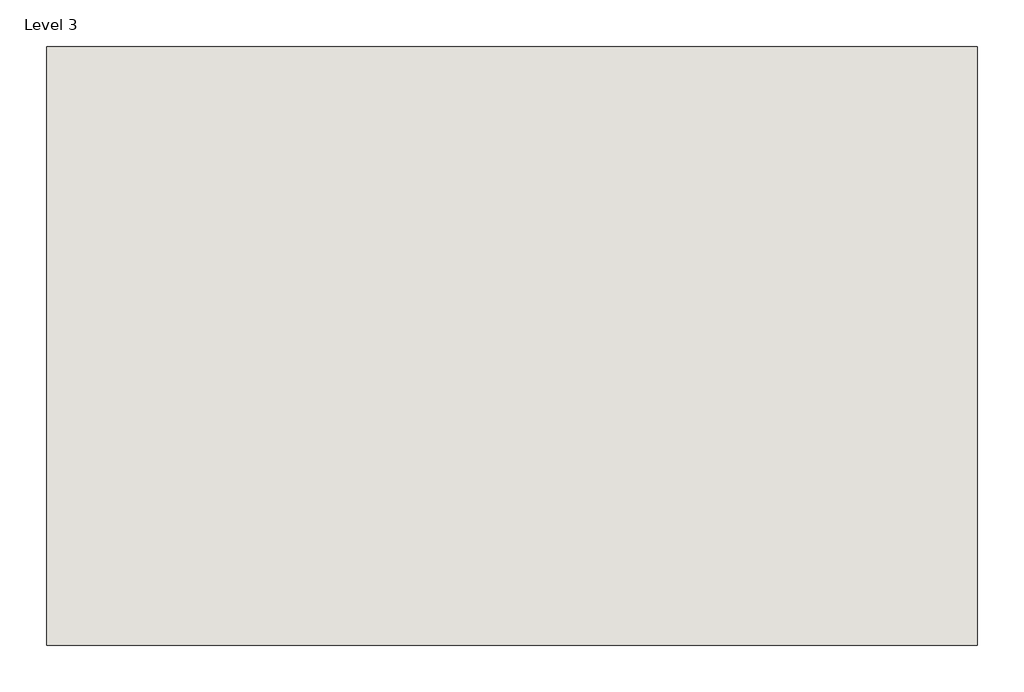
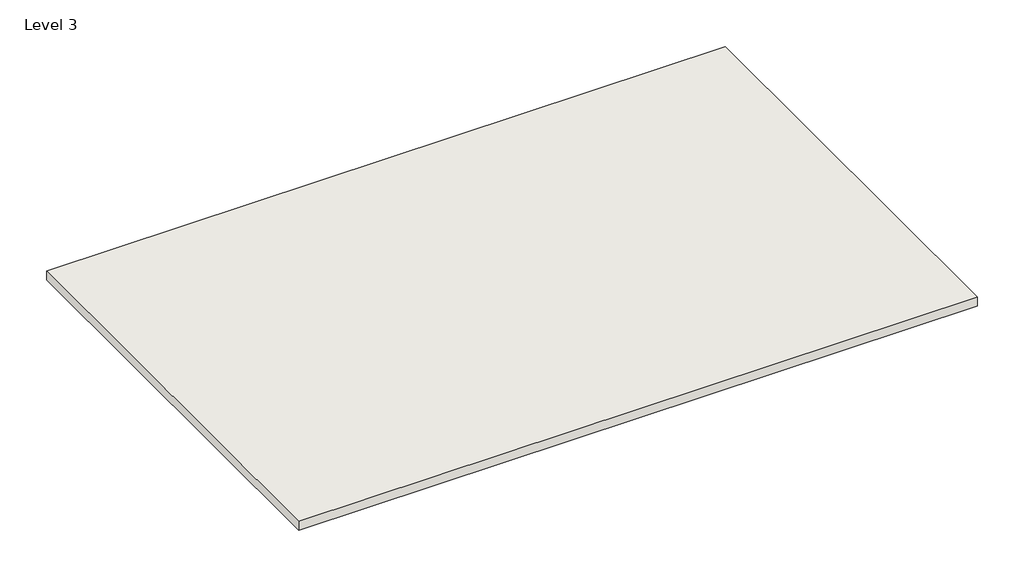
# One storey: 1 wall.
"""IFC4 building model written with IfcOpenShell, lengths in millimetres."""

from ifc_helpers import new_model, si_unit, origin, place, context, project, spatial, transform, mapped, element, save
from components import walls_2_walls_2_982de27e

model = new_model("IFC4")

# Units and contexts
model_context = context("Model", 3, world=origin())
ifc_project = project(units=[si_unit("LENGTHUNIT", "METRE", prefix="MILLI")], contexts=[model_context])

# Site, building, storey
site = spatial("IfcSite", under=ifc_project)
building = spatial("IfcBuilding", under=site)
storey = spatial("IfcBuildingStorey", under=building, Name="Level 3", Elevation=9144.0)

# Wall
placement = place(None, origin())
walls_2_walls_2_shape = walls_2_walls_2_982de27e(model_context)
element("IfcWall", 1, ObjectType="Walls 2 : Walls 2", at=placement, inside=storey, context=model_context, shape_type="MappedRepresentation", body=[
    mapped(walls_2_walls_2_shape, transform((0.0, 0.0, 0.0), x_axis=(1.0, 0.0, 0.0), y_axis=(0.0, 1.0, 0.0), z_axis=(0.0, 0.0, 1.0))),
])

save(model, "model.ifc")

# Revit data of these elements
# Element 1 (IfcWall, "Walls 2 : Walls 2")
#   Phase Created = New Construction
#   Materials on its faces: "Default Wall"
# Materials
#   "Default Wall": colour RGB 80 80 80, transparency 0
